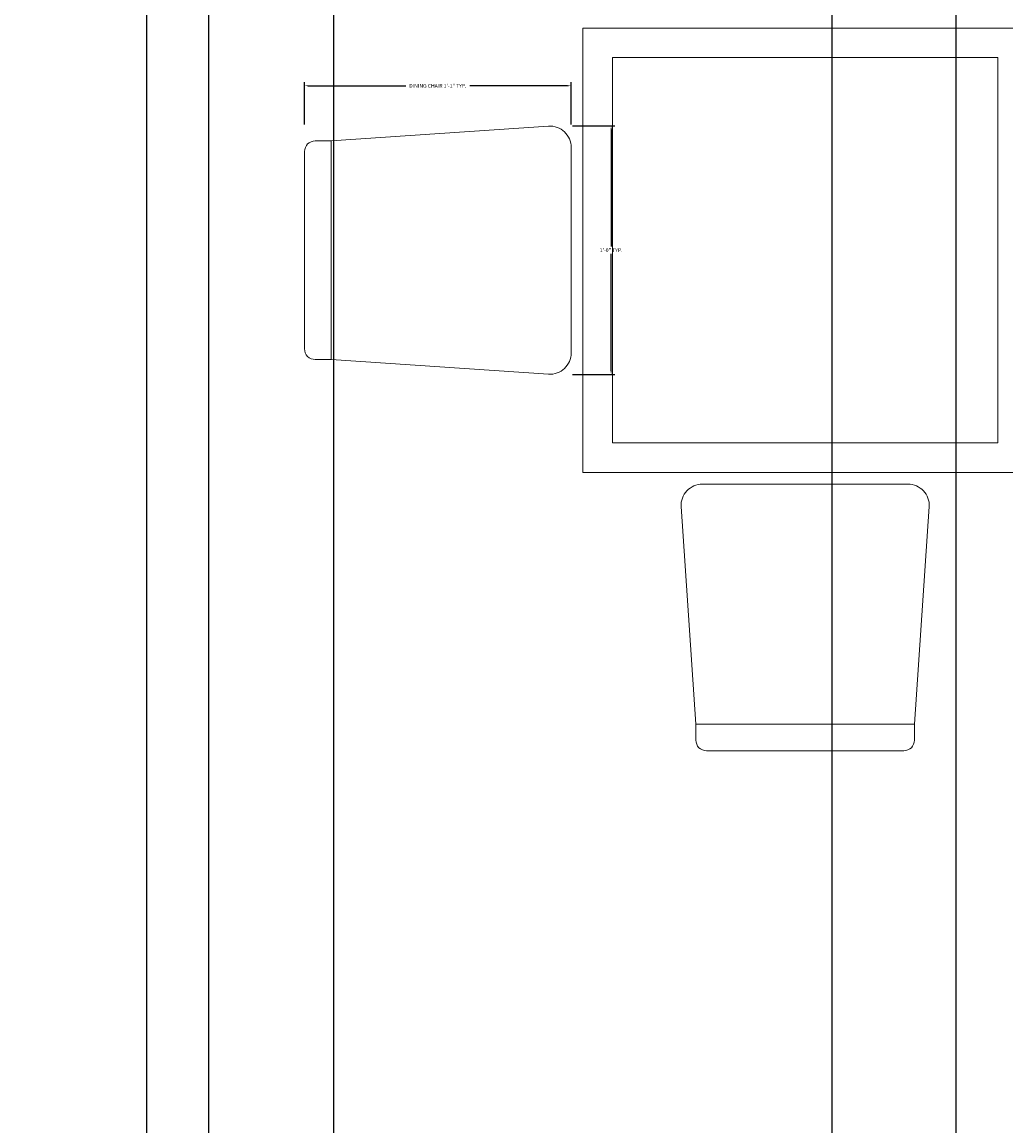
# Model space of a CAD drawing. Units: inches. Extents: x 0 to 281, y -535 to 46.
# Tile 5 of 22: x 150 to 198, y -222 to -168. Entities that reach past the tile are written whole.
import ezdxf

# ---------------------------------------------------------------- set-up
doc = ezdxf.new("R2010")
doc.units = ezdxf.units.IN
doc.header["$MEASUREMENT"] = 0
doc.layers.add('A-ANNO-DIMS', color=2, linetype='Continuous', lineweight=18)
doc.layers.add('A-FURN', color=8, linetype='Continuous', lineweight=18)
doc.styles.get("Standard").update_dxf_attribs({"font": 'arial.ttf'})
doc.dimstyles.get("Standard").update_dxf_attribs({"dimtxt": 0.18, "dimasz": 0.18, "dimexe": 0.18, "dimexo": 0.0625, "dimgap": 0.09, "dimtad": 0, "dimtih": 1, "dimtoh": 1, "dimdec": 0, "dimzin": 0, "dimdsep": 46, "dimlunit": 3, "dimtxsty": 'Standard', "dimcen": 0.09, "dimadec": 0, "dimazin": 0, "dimtfac": 1, "dimtdec": 0, "dimtofl": 0, "dimtmove": 0, "dimatfit": 3, "dimfxl": 1, "dimtolj": 1, "dimtzin": 0, "dimarcsym": 0})

# ---------------------------------------------------------------- blocks, each defined once
blk = doc.blocks.new('CHAIR-DINING')
for p, q in [((10.729, 12.842), (1.225, 12.842)), ((0.712, 12.329), (0.712, 11.558)), ((11.243, 11.558), (11.243, 12.329)), ((0, 1.083), (0.712, 11.558)), ((11.243, 11.558), (0.712, 11.558)), ((11.243, 11.558), (11.954, 1.083)), ((1.026, 0), (10.928, 0))]:
    blk.add_line(p, q)
for centre, radius, start, end in [((1.225, 12.329), 0.514, 90, 180), ((10.729, 12.329), 0.514, 0, 90), ((1.026, 1.027), 1.027, 176.8779, 270), ((10.928, 1.027), 1.027, 270, 3.1221)]:
    blk.add_arc(centre, radius, start, end)
blk = doc.blocks.new('*D26')
at = {"layer": 'A-ANNO-DIMS', "color": 0, "lineweight": -2, "transparency": 16777216}
for p, q in [((164.065, -173.329), (164.065, -171.285)), ((164.245, -171.465), (168.951, -171.465)), ((176.727, -171.465), (172.021, -171.465)), ((176.907, -173.329), (176.907, -171.285))]:
    blk.add_line(p, q, dxfattribs=at)
at = {"layer": 'A-ANNO-DIMS', "color": 0, "transparency": 16777216}
for points in [[(164.245, -171.435), (164.245, -171.495), (164.065, -171.465)], [(176.727, -171.435), (176.727, -171.495), (176.907, -171.465)]]:
    blk.add_solid(points, dxfattribs=at)
at = {"layer": 'Defpoints', "color": 0, "transparency": 16777216}
for p in [(164.065, -171.465), (164.065, -173.392), (176.907, -173.392)]:
    blk.add_point(p, dxfattribs=at)
at = {"layer": 'A-ANNO-DIMS', "color": 0, "transparency": 16777216, "insert": (170.486, -171.465), "char_height": 0.18, "attachment_point": 5}
blk.add_mtext('\\A1;DINING CHAIR 1\'-1" TYP.', dxfattribs=at)
blk = doc.blocks.new('*D27')
at = {"layer": 'A-ANNO-DIMS', "color": 0, "lineweight": -2, "transparency": 16777216}
for p, q in [((176.97, -173.392), (179.014, -173.392)), ((178.834, -173.572), (178.834, -179.202)), ((178.834, -185.196), (178.834, -179.566)), ((176.97, -185.376), (179.014, -185.376))]:
    blk.add_line(p, q, dxfattribs=at)
at = {"layer": 'A-ANNO-DIMS', "color": 0, "transparency": 16777216}
for points in [[(178.804, -173.572), (178.864, -173.572), (178.834, -173.392)], [(178.804, -185.196), (178.864, -185.196), (178.834, -185.376)]]:
    blk.add_solid(points, dxfattribs=at)
at = {"layer": 'Defpoints', "color": 0, "transparency": 16777216}
for p in [(176.907, -173.392), (178.834, -173.392), (176.907, -185.376)]:
    blk.add_point(p, dxfattribs=at)
at = {"layer": 'A-ANNO-DIMS', "color": 0, "transparency": 16777216, "insert": (178.834, -179.384), "char_height": 0.18, "attachment_point": 5}
blk.add_mtext('\\A1;1\'-0" TYP.', dxfattribs=at)
blk = doc.blocks.new('*D41')
at = {"layer": 'A-ANNO-DIMS', "color": 0, "lineweight": -2, "transparency": 16777216}
for p, q in [((120.459, -131.473), (120.459, -535.041)), ((156.459, -131.473), (156.459, -535.041)), ((120.639, -534.861), (138.13, -534.861)), ((156.279, -534.861), (138.788, -534.861))]:
    blk.add_line(p, q, dxfattribs=at)
at = {"layer": 'A-ANNO-DIMS', "color": 0, "transparency": 16777216}
for points in [[(120.639, -534.831), (120.639, -534.891), (120.459, -534.861)], [(156.279, -534.831), (156.279, -534.891), (156.459, -534.861)]]:
    blk.add_solid(points, dxfattribs=at)
at = {"layer": 'Defpoints', "color": 0, "transparency": 16777216}
for p in [(120.459, -131.411), (156.459, -131.411), (156.459, -534.861)]:
    blk.add_point(p, dxfattribs=at)
at = {"layer": 'A-ANNO-DIMS', "color": 0, "transparency": 16777216, "insert": (138.459, -534.861), "char_height": 0.18, "attachment_point": 5}
blk.add_mtext('\\A1;3\'-0"', dxfattribs=at)
blk = doc.blocks.new('*D42')
at = {"layer": 'A-ANNO-DIMS', "color": 0, "lineweight": -2, "transparency": 16777216}
for p, q in [((165.459, -131.473), (165.459, -535.041)), ((189.459, -131.473), (189.459, -535.041)), ((165.639, -534.861), (177.128, -534.861)), ((189.279, -534.861), (177.79, -534.861))]:
    blk.add_line(p, q, dxfattribs=at)
at = {"layer": 'A-ANNO-DIMS', "color": 0, "transparency": 16777216}
for points in [[(165.639, -534.831), (165.639, -534.891), (165.459, -534.861)], [(189.279, -534.831), (189.279, -534.891), (189.459, -534.861)]]:
    blk.add_solid(points, dxfattribs=at)
at = {"layer": 'Defpoints', "color": 0, "transparency": 16777216}
for p in [(165.459, -131.411), (189.459, -131.411), (189.459, -534.861)]:
    blk.add_point(p, dxfattribs=at)
at = {"layer": 'A-ANNO-DIMS', "color": 0, "transparency": 16777216, "insert": (177.459, -534.861), "char_height": 0.18, "attachment_point": 5}
blk.add_mtext('\\A1;2\'-0"', dxfattribs=at)
blk = doc.blocks.new('*D46')
at = {"layer": 'A-ANNO-DIMS', "color": 0, "lineweight": -2, "transparency": 16777216}
for p, q in [((159.459, -263.348), (159.459, 46.219)), ((159.639, 46.039), (177.13, 46.039)), ((195.279, 46.039), (177.788, 46.039)), ((195.459, -263.348), (195.459, 46.219))]:
    blk.add_line(p, q, dxfattribs=at)
at = {"layer": 'A-ANNO-DIMS', "color": 0, "transparency": 16777216}
for points in [[(159.639, 46.069), (159.639, 46.009), (159.459, 46.039)], [(195.279, 46.069), (195.279, 46.009), (195.459, 46.039)]]:
    blk.add_solid(points, dxfattribs=at)
at = {"layer": 'Defpoints', "color": 0, "transparency": 16777216}
for p in [(195.459, 46.039), (159.459, -263.411), (195.459, -263.411)]:
    blk.add_point(p, dxfattribs=at)
at = {"layer": 'A-ANNO-DIMS', "color": 0, "transparency": 16777216, "insert": (177.459, 46.039), "char_height": 0.18, "attachment_point": 5}
blk.add_mtext('\\A1;3\'-0"', dxfattribs=at)
blk = doc.blocks.new('*D48')
at = {"layer": 'A-ANNO-DIMS', "color": 0, "lineweight": -2, "transparency": 16777216}
for p, q in [((159.459, -392.348), (159.459, 46.219)), ((159.639, 46.039), (177.13, 46.039)), ((195.279, 46.039), (177.788, 46.039)), ((195.459, -392.348), (195.459, 46.219))]:
    blk.add_line(p, q, dxfattribs=at)
at = {"layer": 'A-ANNO-DIMS', "color": 0, "transparency": 16777216}
for points in [[(159.639, 46.069), (159.639, 46.009), (159.459, 46.039)], [(195.279, 46.069), (195.279, 46.009), (195.459, 46.039)]]:
    blk.add_solid(points, dxfattribs=at)
at = {"layer": 'Defpoints', "color": 0, "transparency": 16777216}
for p in [(195.459, 46.039), (159.459, -392.411), (195.459, -392.411)]:
    blk.add_point(p, dxfattribs=at)
at = {"layer": 'A-ANNO-DIMS', "color": 0, "transparency": 16777216, "insert": (177.459, 46.039), "char_height": 0.18, "attachment_point": 5}
blk.add_mtext('\\A1;3\'-0"', dxfattribs=at)

msp = doc.modelspace()

# ---------------------------------------------------------------- linework, layer by layer
at = {"layer": 'A-FURN'}
for points in [[(177.478, -190.086), (177.478, -168.682), (198.882, -168.682), (198.882, -190.086)], [(178.905, -188.659), (178.905, -170.109), (197.455, -170.109), (197.455, -188.659)]]:
    msp.add_lwpolyline(points, close=True, dxfattribs=at)

# ---------------------------------------------------------------- block references
for p, rotation in [((176.907, -185.361), 90.00000000119184), ((194.157, -190.656), 180)]:
    msp.add_blockref('CHAIR-DINING', p, dxfattribs=dict(at, rotation=rotation))

# ---------------------------------------------------------------- dimensions: what is measured, and where the dimension line sits
at = {"layer": 'A-ANNO-DIMS'}
for base, p1, p2, picture, middle in [((195.459, 46.039), (159.459, -263.411), (195.459, -263.411), '*D46', (177.459, 46.039)), ((195.459, 46.039), (159.459, -392.411), (195.459, -392.411), '*D48', (177.459, 46.039)), ((156.459, -534.861), (120.459, -131.411), (156.459, -131.411), '*D41', (138.459, -534.861)), ((189.459, -534.861), (165.459, -131.411), (189.459, -131.411), '*D42', (177.459, -534.861))]:
    dim = msp.add_linear_dim(base=base, p1=p1, p2=p2, dimstyle='Standard', override={"dimdec": 1, "dimlfac": 1, "dimrnd": 0, "dimzin": 1, "dimdsep": 46, "dimlunit": 4, "dimfrac": 2}, dxfattribs=at)
    dim.commit()
    dim.dimension.update_dxf_attribs({"geometry": picture, "text_midpoint": middle})
for base, p1, p2, angle, text, picture, middle in [((164.065, -171.465), (176.907, -173.392), (164.065, -173.392), 180, 'DINING CHAIR <> TYP.', '*D26', (170.486, -171.465)), ((178.834, -173.392), (176.907, -185.376), (176.907, -173.392), 90, '<> TYP.', '*D27', (178.834, -179.384))]:
    dim = msp.add_linear_dim(base=base, p1=p1, p2=p2, angle=angle, text=text, dimstyle='Standard', override={"dimdec": 1, "dimlfac": 1, "dimrnd": 0, "dimzin": 1, "dimdsep": 46, "dimlunit": 4, "dimfrac": 2}, dxfattribs=at)
    dim.commit()
    dim.dimension.update_dxf_attribs({"geometry": picture, "text_midpoint": middle})

doc.saveas('drawing.dxf')
